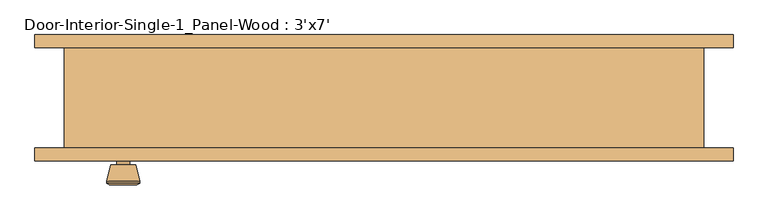
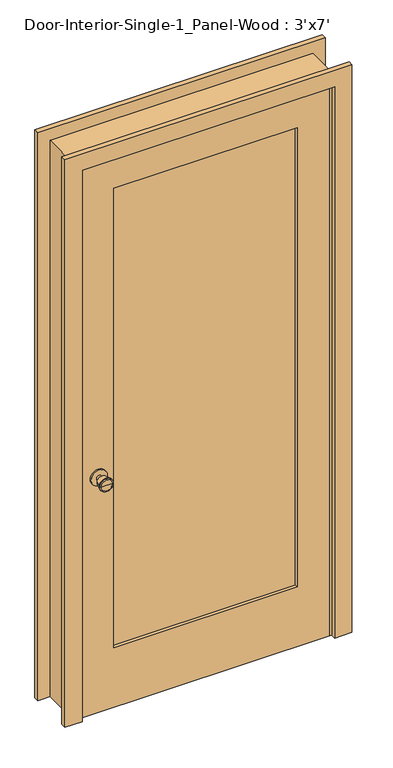
"""IFC4 building model written with IfcOpenShell, lengths in millimetres: door geometry, Door-Interior-Single-1_Panel-Wood : 3'x7'."""

from ifc_helpers import new_model, si_unit, point, frame, frame_2d, origin, place, context, project, spatial, polyline, circle_curve, trimmed, segment, composite_curve, outline, extrude, faceted_brep, source, transform, mapped, element, save
from ifc_brep_helpers import plane_surface, cylinder_surface, revolved_surface, advanced_brep


def door_interior_single_1_panel_wood_3_x7_5a860750(model_context):
    return source(origin(), model_context, "Body", "SolidModel", [
        advanced_brep(
        [(-393.7, -32.1, 914.4), (-403.7, -32.1, 914.4), (-383.7, -32.1, 914.4), (-373.2241324, 16.9, 914.4), (-414.1758676, 16.9, 914.4), (-393.7, 16.9, 914.4), (-368.7, 15.0721319, 914.4), (-418.7, 15.0721319, 914.4), (-368.7, 11.6084537, 914.4), (-418.7, 11.6084537, 914.4), (-375.063764, -13.1, 914.4), (-412.336236, -13.1, 914.4), (-383.7, -13.1, 914.4), (-403.7, -13.1, 914.4)],
        [
            (0, 1),
            (1, 2, circle_curve(frame((-393.7, -32.1, 914.4), z_axis=(0.0, -1.0, 0.0), x_axis=(-1.0, 0.0, 0.0)), 10.0)),
            (2, 0),
            (2, 1, circle_curve(frame((-393.7, -32.1, 914.4), z_axis=(0.0, -1.0, 0.0), x_axis=(-1.0, 0.0, 0.0)), 10.0)),
            (3, 4, circle_curve(frame((-393.7, 16.9, 914.4), z_axis=(0.0, 1.0, 0.0), x_axis=(-1.0, 0.0, 0.0)), 20.4758676)),
            (4, 5),
            (5, 3),
            (4, 3, circle_curve(frame((-393.7, 16.9, 914.4), z_axis=(0.0, 1.0, 0.0), x_axis=(-1.0, 0.0, 0.0)), 20.4758676)),
            (6, 7, circle_curve(frame((-393.7, 15.0721319, 914.4), z_axis=(0.0, 1.0, 0.0), x_axis=(-1.0, 0.0, 0.0)), 25.0)),
            (7, 4),
            (3, 6),
            (7, 6, circle_curve(frame((-393.7, 15.0721319, 914.4), z_axis=(0.0, 1.0, 0.0), x_axis=(-1.0, 0.0, 0.0)), 25.0)),
            (8, 9, circle_curve(frame((-393.7, 11.6084537, 914.4), z_axis=(0.0, 1.0, 0.0), x_axis=(-1.0, 0.0, 0.0)), 25.0)),
            (9, 7),
            (6, 8),
            (9, 8, circle_curve(frame((-393.7, 11.6084537, 914.4), z_axis=(0.0, 1.0, 0.0), x_axis=(-1.0, 0.0, 0.0)), 25.0)),
            (10, 11, circle_curve(frame((-393.7, -13.1, 914.4), z_axis=(0.0, 1.0, 0.0), x_axis=(-1.0, 0.0, 0.0)), 18.636236)),
            (11, 9),
            (8, 10),
            (11, 10, circle_curve(frame((-393.7, -13.1, 914.4), z_axis=(0.0, 1.0, 0.0), x_axis=(-1.0, 0.0, 0.0)), 18.636236)),
            (12, 13, circle_curve(frame((-393.7, -13.1, 914.4), z_axis=(0.0, 1.0, 0.0), x_axis=(-1.0, 0.0, 0.0)), 10.0)),
            (13, 11),
            (10, 12),
            (13, 12, circle_curve(frame((-393.7, -13.1, 914.4), z_axis=(0.0, 1.0, 0.0), x_axis=(-1.0, 0.0, 0.0)), 10.0)),
            (1, 13),
            (12, 2),
        ],
        [
            plane_surface(frame((-393.7, -32.1, 914.4), z_axis=(0.0, -1.0, 0.0), x_axis=(-1.0, 0.0, 0.0))),
            plane_surface(frame((-393.7, 16.9, 914.4), z_axis=(0.0, 1.0, 0.0), x_axis=(-1.0, 0.0, 0.0))),
            revolved_surface(polyline([(-414.1758676, 16.9, 914.4), (-418.7, 15.0721319, 914.4)]), (-393.7, -32.1, 914.4), (0.0, -1.0, 0.0)),
            cylinder_surface(frame((-393.7, -32.1, 914.4), z_axis=(0.0, -1.0, 0.0), x_axis=(-1.0, 0.0, 0.0)), 25.0),
            revolved_surface(polyline([(-418.7, 11.6084537, 914.4), (-412.336236, -13.1, 914.4)]), (-393.7, -32.1, 914.4), (0.0, -1.0, 0.0)),
            plane_surface(frame((-393.7, -13.1, 914.4), z_axis=(0.0, -1.0, 0.0), x_axis=(-1.0, 0.0, 0.0))),
            cylinder_surface(frame((-393.7, -32.1, 914.4), z_axis=(0.0, -1.0, 0.0), x_axis=(-1.0, 0.0, 0.0)), 10.0),
        ],
        [
            (0, [[1, 2, 3]]),
            (0, [[-3, 4, -1]]),
            (1, [[5, 6, 7]]),
            (1, [[8, -7, -6]]),
            (2, [[9, 10, -5, 11]]),
            (2, [[12, -11, -8, -10]]),
            (3, [[13, 14, -9, 15]]),
            (3, [[16, -15, -12, -14]]),
            (4, [[17, 18, -13, 19]]),
            (4, [[20, -19, -16, -18]]),
            (5, [[21, 22, -17, 23]]),
            (5, [[24, -23, -20, -22]]),
            (6, [[-2, 25, -21, 26]]),
            (6, [[-4, -26, -24, -25]]),
        ],
    ),
        extrude(outline(composite_curve([segment(trimmed(circle_curve(frame_2d((914.4, -393.7)), 30.0), [point((914.4, -423.7))], [point((914.4, -363.7))], False, "CARTESIAN"), True, "CONTINUOUS"), segment(trimmed(circle_curve(frame_2d((914.4, -393.7)), 30.0), [point((914.4, -363.7))], [point((914.4, -423.7))], False, "CARTESIAN"), True, "CONTINUOUS")], self_intersect=False)), frame((0.0, -38.1, 0.0), z_axis=(0.0, 1.0, 0.0), x_axis=(0.0, 0.0, 1.0)), (0.0, 0.0, 1.0), 6.0),
        advanced_brep(
        [(-393.7, -79.025, 914.4), (-383.7, -79.025, 914.4), (-403.7, -79.025, 914.4), (-373.2241324, -128.025, 914.4), (-393.7, -128.025, 914.4), (-414.1758676, -128.025, 914.4), (-368.7, -126.1971319, 914.4), (-418.7, -126.1971319, 914.4), (-368.7, -122.7334537, 914.4), (-418.7, -122.7334537, 914.4), (-375.063764, -98.025, 914.4), (-412.336236, -98.025, 914.4), (-383.7, -98.025, 914.4), (-403.7, -98.025, 914.4)],
        [
            (0, 1),
            (1, 2, circle_curve(frame((-393.7, -79.025, 914.4), z_axis=(0.0, 1.0, 0.0), x_axis=(-1.0, 0.0, 0.0)), 10.0)),
            (2, 0),
            (2, 1, circle_curve(frame((-393.7, -79.025, 914.4), z_axis=(0.0, 1.0, 0.0), x_axis=(-1.0, 0.0, 0.0)), 10.0)),
            (3, 4),
            (4, 5),
            (5, 3, circle_curve(frame((-393.7, -128.025, 914.4), z_axis=(0.0, -1.0, 0.0), x_axis=(-1.0, 0.0, 0.0)), 20.4758676)),
            (3, 5, circle_curve(frame((-393.7, -128.025, 914.4), z_axis=(0.0, -1.0, 0.0), x_axis=(-1.0, 0.0, 0.0)), 20.4758676)),
            (6, 3),
            (5, 7),
            (7, 6, circle_curve(frame((-393.7, -126.1971319, 914.4), z_axis=(0.0, -1.0, 0.0), x_axis=(-1.0, 0.0, 0.0)), 25.0)),
            (6, 7, circle_curve(frame((-393.7, -126.1971319, 914.4), z_axis=(0.0, -1.0, 0.0), x_axis=(-1.0, 0.0, 0.0)), 25.0)),
            (8, 6),
            (7, 9),
            (9, 8, circle_curve(frame((-393.7, -122.7334537, 914.4), z_axis=(0.0, -1.0, 0.0), x_axis=(-1.0, 0.0, 0.0)), 25.0)),
            (8, 9, circle_curve(frame((-393.7, -122.7334537, 914.4), z_axis=(0.0, -1.0, 0.0), x_axis=(-1.0, 0.0, 0.0)), 25.0)),
            (10, 8),
            (9, 11),
            (11, 10, circle_curve(frame((-393.7, -98.025, 914.4), z_axis=(0.0, -1.0, 0.0), x_axis=(-1.0, 0.0, 0.0)), 18.636236)),
            (10, 11, circle_curve(frame((-393.7, -98.025, 914.4), z_axis=(0.0, -1.0, 0.0), x_axis=(-1.0, 0.0, 0.0)), 18.636236)),
            (12, 10),
            (11, 13),
            (13, 12, circle_curve(frame((-393.7, -98.025, 914.4), z_axis=(0.0, -1.0, 0.0), x_axis=(-1.0, 0.0, 0.0)), 10.0)),
            (12, 13, circle_curve(frame((-393.7, -98.025, 914.4), z_axis=(0.0, -1.0, 0.0), x_axis=(-1.0, 0.0, 0.0)), 10.0)),
            (1, 12),
            (13, 2),
        ],
        [
            plane_surface(frame((-393.7, -79.025, 914.4), z_axis=(0.0, 1.0, 0.0), x_axis=(-1.0, 0.0, 0.0))),
            plane_surface(frame((-393.7, -128.025, 914.4), z_axis=(0.0, -1.0, 0.0), x_axis=(-1.0, 0.0, 0.0))),
            revolved_surface(polyline([(-414.1758676, -128.025, 914.4), (-418.7, -126.1971319, 914.4)]), (-393.7, -79.025, 914.4), (0.0, 1.0, 0.0)),
            cylinder_surface(frame((-393.7, -79.025, 914.4), z_axis=(0.0, 1.0, 0.0), x_axis=(-1.0, 0.0, 0.0)), 25.0),
            revolved_surface(polyline([(-418.7, -122.7334537, 914.4), (-412.336236, -98.025, 914.4)]), (-393.7, -79.025, 914.4), (0.0, 1.0, 0.0)),
            plane_surface(frame((-393.7, -98.025, 914.4), z_axis=(0.0, 1.0, 0.0), x_axis=(-1.0, 0.0, 0.0))),
            cylinder_surface(frame((-393.7, -79.025, 914.4), z_axis=(0.0, 1.0, 0.0), x_axis=(-1.0, 0.0, 0.0)), 10.0),
        ],
        [
            (0, [[1, 2, 3]]),
            (0, [[-3, 4, -1]]),
            (1, [[5, 6, 7]]),
            (1, [[-6, -5, 8]]),
            (2, [[9, -7, 10, 11]]),
            (2, [[-10, -8, -9, 12]]),
            (3, [[13, -11, 14, 15]]),
            (3, [[-14, -12, -13, 16]]),
            (4, [[17, -15, 18, 19]]),
            (4, [[-18, -16, -17, 20]]),
            (5, [[21, -19, 22, 23]]),
            (5, [[-22, -20, -21, 24]]),
            (6, [[25, -23, 26, -2]]),
            (6, [[-26, -24, -25, -4]]),
        ],
    ),
        extrude(outline(composite_curve([segment(trimmed(circle_curve(frame_2d((914.4, -393.7)), 30.0), [point((914.4, -423.7))], [point((914.4, -363.7))], False, "CARTESIAN"), True, "CONTINUOUS"), segment(trimmed(circle_curve(frame_2d((914.4, -393.7)), 30.0), [point((914.4, -363.7))], [point((914.4, -423.7))], False, "CARTESIAN"), True, "CONTINUOUS")], self_intersect=False)), frame((0.0, -79.025, 0.0), z_axis=(0.0, 1.0, 0.0), x_axis=(0.0, 0.0, 1.0)), (0.0, 0.0, 1.0), 6.0),
        faceted_brep([(482.6, -73.025, 0.0), (457.2, -73.025, 0.0), (457.2, -38.1, 0.0), (444.5, -38.1, 0.0), (444.5, -3.175, 0.0), (457.2, -3.175, 0.0), (457.2, 79.375, 0.0), (482.6, 79.375, 0.0), (482.6, 79.375, 2159.0), (482.6, -73.025, 2159.0), (457.2, 79.375, 2133.6), (-457.2, 79.375, 2133.6), (-457.2, 79.375, 0.0), (-482.6, 79.375, 0.0), (-482.6, 79.375, 2159.0), (457.2, -3.175, 2133.6), (444.5, -3.175, 2120.9), (-444.5, -3.175, 2120.9), (-444.5, -3.175, 0.0), (-457.2, -3.175, 0.0), (-457.2, -3.175, 2133.6), (444.5, -38.1, 2120.9), (457.2, -38.1, 2133.6), (-457.2, -38.1, 2133.6), (-457.2, -38.1, 0.0), (-444.5, -38.1, 0.0), (-444.5, -38.1, 2120.9), (457.2, -73.025, 2133.6), (-482.6, -73.025, 2159.0), (-482.6, -73.025, 0.0), (-457.2, -73.025, 0.0), (-457.2, -73.025, 2133.6)], [[[0, 1, 2, 3, 4, 5, 6, 7]], [[7, 8, 9, 0]], [[6, 10, 11, 12, 13, 14, 8, 7]], [[5, 15, 10, 6]], [[4, 16, 17, 18, 19, 20, 15, 5]], [[3, 21, 16, 4]], [[2, 22, 23, 24, 25, 26, 21, 3]], [[1, 27, 22, 2]], [[0, 9, 28, 29, 30, 31, 27, 1]], [[8, 14, 28, 9]], [[15, 20, 11, 10]], [[21, 26, 17, 16]], [[27, 31, 23, 22]], [[29, 13, 12, 19, 18, 25, 24, 30]], [[14, 13, 29, 28]], [[20, 19, 12, 11]], [[26, 25, 18, 17]], [[31, 30, 24, 23]]]),
        extrude(outline(polyline([(2133.6, -457.2), (0.0, -457.2), (0.0, 457.2), (2133.6, 457.2), (2133.6, -457.2)]), holes=[polyline([(2014.5375, -336.55), (2014.5375, 336.55), (231.775, 336.55), (231.775, -336.55), (2014.5375, -336.55)])]), frame((0.0, -73.025, 0.0), z_axis=(0.0, 1.0, 0.0), x_axis=(0.0, 0.0, 1.0)), (0.0, 0.0, 1.0), 34.925),
        extrude(outline(polyline([(336.55, -49.7416667), (336.55, -61.3833333), (-336.55, -61.3833333), (-336.55, -49.7416667), (336.55, -49.7416667)])), frame((0.0, 0.0, 231.775), z_axis=(0.0, 0.0, 1.0), x_axis=(1.0, 0.0, 0.0)), (0.0, 0.0, 1.0), 1782.7625),
        extrude(outline(polyline([(0.0, 527.05), (2203.45, 527.05), (2203.45, -527.05), (0.0, -527.05), (0.0, -463.55), (2139.95, -463.55), (2139.95, 463.55), (0.0, 463.55), (0.0, 527.05)])), frame((0.0, -92.075, 0.0), z_axis=(0.0, 1.0, 0.0), x_axis=(0.0, 0.0, 1.0)), (0.0, 0.0, 1.0), 19.05),
        extrude(outline(polyline([(0.0, 527.05), (2203.45, 527.05), (2203.45, -527.05), (0.0, -527.05), (0.0, -463.55), (2139.95, -463.55), (2139.95, 463.55), (0.0, 463.55), (0.0, 527.05)])), frame((0.0, 79.375, 0.0), z_axis=(0.0, 1.0, 0.0), x_axis=(0.0, 0.0, 1.0)), (0.0, 0.0, 1.0), 19.05),
    ])


if __name__ == "__main__":
    model = new_model("IFC4")
    model_context = context("Model", 3, world=origin())
    ifc_project = project(units=[si_unit("LENGTHUNIT", "METRE", prefix="MILLI")], contexts=[model_context])
    site = spatial("IfcSite", under=ifc_project)
    building = spatial("IfcBuilding", under=site)
    placement = place(None, origin())
    door_interior_single_1_panel_wood_3_x7_shape = door_interior_single_1_panel_wood_3_x7_5a860750(model_context)
    element("IfcDoor", 1, ObjectType="Door-Interior-Single-1_Panel-Wood : 3'x7'", at=placement, inside=building, context=model_context, shape_type="MappedRepresentation", body=[
        mapped(door_interior_single_1_panel_wood_3_x7_shape, transform((0.0, 0.0, 0.0), x_axis=(1.0, 0.0, 0.0), y_axis=(0.0, 1.0, 0.0), z_axis=(0.0, 0.0, 1.0))),
    ])
    save(model, "model.ifc")

# Revit data of these elements
# Type "Door-Interior-Single-1_Panel-Wood : 3'x7'"
#   Type Mark = "9"
#   Assembly Code = "C1020300"
#   Analytic Construction = "Wooden"
#   Top Rail = 0' - 4 11/16"
#   Thickness = 0' - 1 3/8"
#   Thermal Resistance (R) = 2.5876 (h·ft²·°F)/BTU
#   Swing Angle [instance default] = 90.00°
#   Stiles = 0' - 4 3/4"
#   Rough Width = 3' - 2"
#   Rough Height = 7' - 1"
#   Height = 7' - 0"
#   Width = 3' - 0"
#   Heat Transfer Coefficient (U) = 0.3865 BTU/(h·ft²·°F)
#   Bottom Rail = 0' - 9 1/8"
#   Trim Material = Cherry
#   Panel Material = Cherry
#   Frame Material = Cherry
#   Door Handle Material = Aluminum
#   Visual Light Transmittance = 0
#   Solar Heat Gain Coefficient = 0
#   Wall Closure = (empty or 0)
#   Function = (empty or 0)
# Element 1 (IfcDoor, "Door-Interior-Single-1_Panel-Wood : 3'x7'")
#   Materials on its faces: "Cherry", "Aluminum"
# Materials
#   "Cherry": class "Wood", colour RGB 226 177 128, transparency 0, Description = "Prunus Serotina", Cost = 0
#   "Aluminum": class "Metal", colour RGB 247 247 247, transparency 0, Description = "Aluminum 6061", Cost = 0
